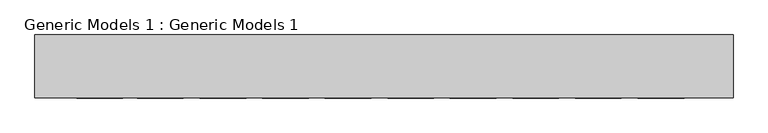
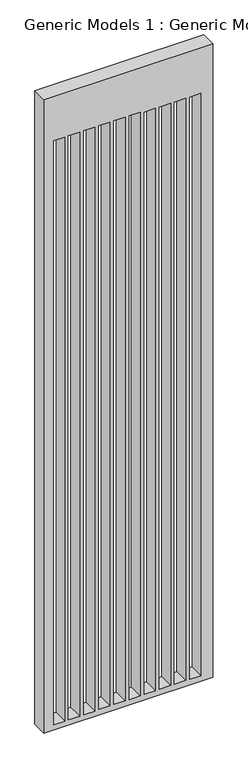
"""IFC4 building model written with IfcOpenShell, lengths in millimetres: proxy geometry, Generic Models 1 : Generic Models 1."""

from ifc_helpers import new_model, si_unit, frame, origin, place, context, project, spatial, polyline, outline, extrude, source, transform, mapped, element, save


def generic_models_1_generic_models_1_2151a878(model_context):
    return source(origin(), model_context, "Body", "SweptSolid", [
        extrude(outline(polyline([(13361.884035, -6448.4108866), (-104.4847331, -6448.4108866), (-104.4847331, -3049.8925988), (13361.884035, -3049.8925988), (13361.884035, -6448.4108866)]), holes=[polyline([(12413.7349672, -6019.9542501), (0.0, -6019.9542501), (0.0, -6245.2108866), (12413.7349672, -6245.2108866), (12413.7349672, -6019.9542501)]), polyline([(12413.4898795, -5725.5400582), (4.3397796, -5725.5400582), (4.3397796, -5950.7966947), (12413.4898795, -5950.7966947), (12413.4898795, -5725.5400582)]), polyline([(12413.4898795, -5420.7400582), (4.7092991, -5420.7400582), (4.7092991, -5645.9966947), (12413.4898795, -5645.9966947), (12413.4898795, -5420.7400582)]), polyline([(12413.4898795, -5115.9400582), (12.5258728, -5115.9400582), (12.5258728, -5341.1966947), (12413.4898795, -5341.1966947), (12413.4898795, -5115.9400582)]), polyline([(12413.4898795, -4811.1400582), (9.2477148, -4811.1400582), (9.2477148, -5036.3966947), (12413.4898795, -5036.3966947), (12413.4898795, -4811.1400582)]), polyline([(12413.4898795, -4506.3400582), (5.9695569, -4506.3400582), (5.9695569, -4731.5966947), (12413.4898795, -4731.5966947), (12413.4898795, -4506.3400582)]), polyline([(12386.9248091, -4202.6999143), (11.4348851, -4202.6999143), (11.4348851, -4427.9565507), (12386.9248091, -4427.9565507), (12386.9248091, -4202.6999143)]), polyline([(12386.9248091, -3897.8999143), (16.6012189, -3897.8999143), (16.6012189, -4123.1565507), (12386.9248091, -4123.1565507), (12386.9248091, -3897.8999143)]), polyline([(12386.9248091, -3593.0999143), (14.5723312, -3593.0999143), (14.5723312, -3818.3565507), (12386.9248091, -3818.3565507), (12386.9248091, -3593.0999143)]), polyline([(12386.9248091, -3288.2999143), (10.1450364, -3288.2999143), (10.1450364, -3513.5565507), (12386.9248091, -3513.5565507), (12386.9248091, -3288.2999143)])]), frame((0.0, -8574.6600272, 0.0), z_axis=(0.0, 1.0, 0.0), x_axis=(0.0, 0.0, 1.0)), (0.0, 0.0, 1.0), 304.8),
    ])


if __name__ == "__main__":
    model = new_model("IFC4")
    model_context = context("Model", 3, world=origin())
    ifc_project = project(units=[si_unit("LENGTHUNIT", "METRE", prefix="MILLI")], contexts=[model_context])
    site = spatial("IfcSite", under=ifc_project)
    building = spatial("IfcBuilding", under=site)
    placement = place(None, origin())
    generic_models_1_generic_models_1_shape = generic_models_1_generic_models_1_2151a878(model_context)
    element("IfcBuildingElementProxy", 1, Name="Generic Models 1 : Generic Models 1", ObjectType="Generic Models 1 : Generic Models 1", at=placement, inside=building, context=model_context, shape_type="MappedRepresentation", body=[
        mapped(generic_models_1_generic_models_1_shape, transform((0.0, 0.0, 0.0), x_axis=(1.0, 0.0, 0.0), y_axis=(0.0, 1.0, 0.0), z_axis=(0.0, 0.0, 1.0))),
    ])
    save(model, "model.ifc")

# Revit data of these elements
# Element 1 (IfcBuildingElementProxy, "Generic Models 1 : Generic Models 1")
#   Materials on its faces: "Doors - Glazing Bars", "Earth"
# Materials
#   "Doors - Glazing Bars": colour RGB 158 107 65, transparency 0
#   "Earth": class "Generic", colour RGB 97 75 62, transparency 0, Description = "Soil", Cost = 0
